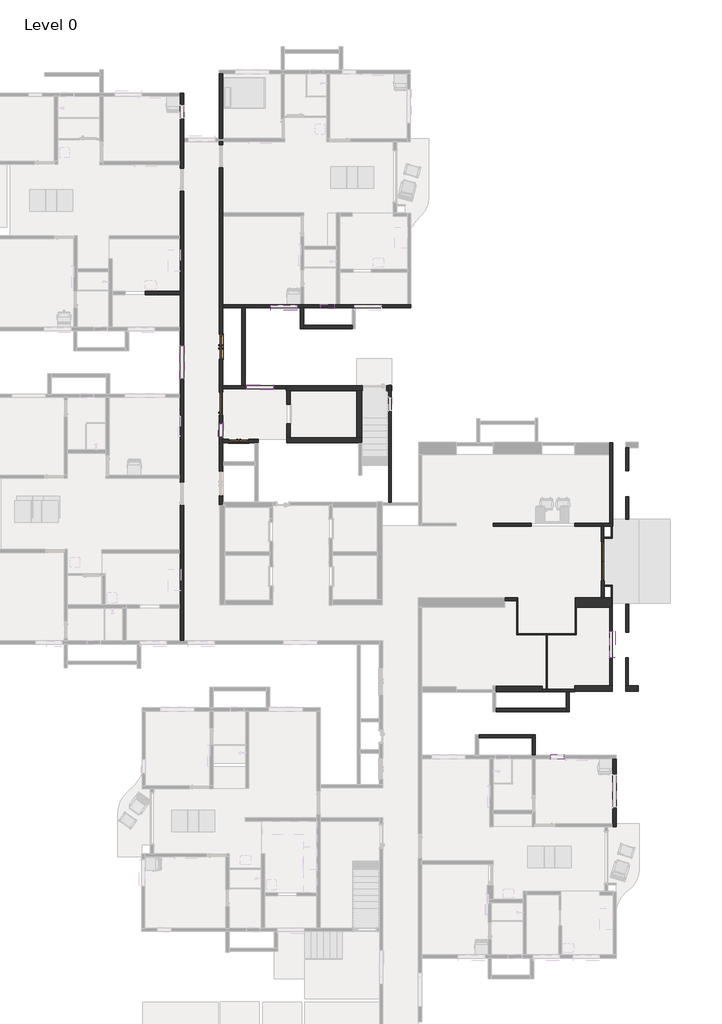
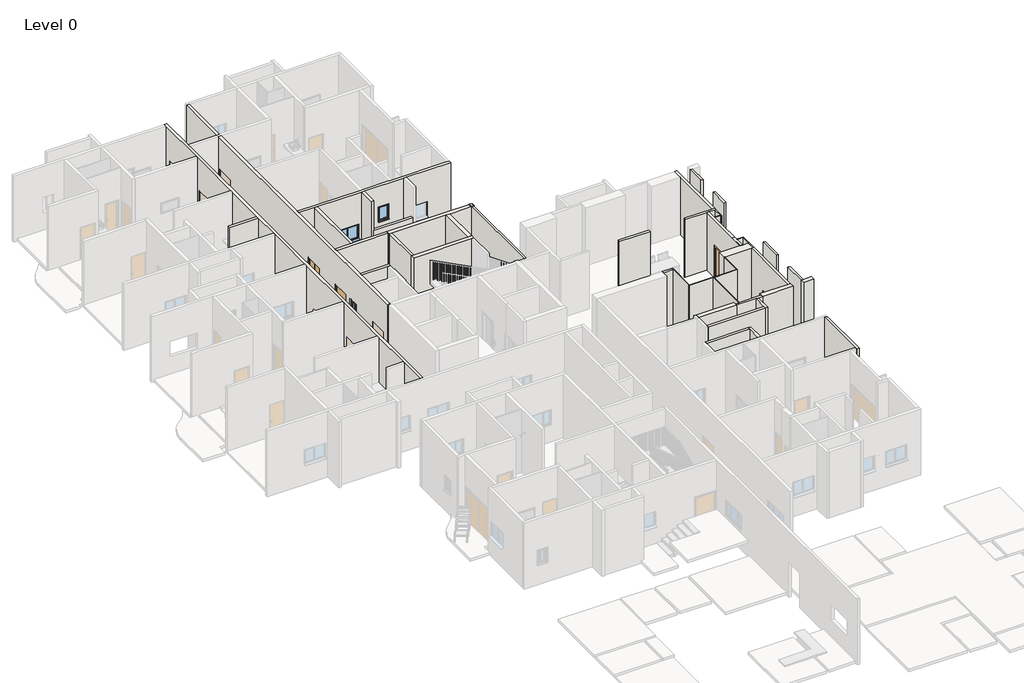
# One storey, part 6 of 14: 43 walls, 7 windows, 4 doors.
"""IFC4 building model written with IfcOpenShell, lengths in millimetres."""

from ifc_helpers import new_model, si_unit, frame, origin, origin_with_axes, place, context, project, spatial, polyline, outline, extrude, faceted_brep, transform, mapped, element, save
from components import doors_extdbl_flush_1810x2110mm_47ab578d, doors_extdbl_flush_3_b8e651f3, doors_extdbl_flush_3_75_39ca422f, doors_extsgl_flush_d1_30a970b5, windows_concept_plain_dbl_4_d1e2e333, windows_concept_plain_dbl_4_70a487c4, windows_sgl_plain_2_be143095, windows_tpl_variable_casement_2_47b04551, windows_tpl_variable_casement_4_346b9f46, windows_tpl_variable_casement_5_ffad3fa3

model = new_model("IFC4")

# Units and contexts
model_context = context("Model", 3, world=origin())
ifc_project = project(units=[si_unit("LENGTHUNIT", "METRE", prefix="MILLI")], contexts=[model_context])

# Site, building, storey
site = spatial("IfcSite", under=ifc_project)
building = spatial("IfcBuilding", under=site)
storey = spatial("IfcBuildingStorey", under=building, Name="Level 0", Elevation=0.0)

# Doors
placement = place(None, origin())
doors_extdbl_flush_1810x2110mm_shape = doors_extdbl_flush_1810x2110mm_47ab578d(model_context)
element("IfcDoor", 1, ObjectType="Doors_ExtDbl_Flush : 1810x2110mm", at=placement, inside=storey, context=model_context, shape_type="MappedRepresentation", body=[
    mapped(doors_extdbl_flush_1810x2110mm_shape, transform((-11411.1602598, 42923.0397358, 355.6), x_axis=(0.0, 1.0, 0.0), y_axis=(-1.0, 0.0, 0.0), z_axis=(0.0, 0.0, 1.0))),
])
doors_extdbl_flush_3_shape = doors_extdbl_flush_3_b8e651f3(model_context)
element("IfcDoor", 2, ObjectType="Doors_ExtDbl_Flush : 3'", at=placement, inside=storey, context=model_context, shape_type="MappedRepresentation", body=[
    mapped(doors_extdbl_flush_3_shape, transform((-28269.1280109, 48493.8706597, 0.0), x_axis=(-1.0, 0.0, 0.0), y_axis=(0.0, -1.0, 0.0), z_axis=(0.0, 0.0, 1.0))),
])
doors_extdbl_flush_3_75_shape = doors_extdbl_flush_3_75_39ca422f(model_context)
element("IfcDoor", 3, ObjectType="Doors_ExtDbl_Flush : 3.75'", at=placement, inside=storey, context=model_context, shape_type="MappedRepresentation", body=[
    mapped(doors_extdbl_flush_3_75_shape, transform((-29094.6788109, 52859.4702597, 0.0), x_axis=(0.0, -1.0, 0.0), y_axis=(1.0, 0.0, 0.0), z_axis=(0.0, 0.0, 1.0))),
])
doors_extsgl_flush_d1_shape = doors_extsgl_flush_d1_30a970b5(model_context)
element("IfcDoor", 4, ObjectType="Doors_ExtSgl_Flush : D1", at=placement, inside=storey, context=model_context, shape_type="MappedRepresentation", body=[
    mapped(doors_extsgl_flush_d1_shape, transform((-29094.6788109, 50221.0706597, 0.0), x_axis=(0.0, 1.0, 0.0), y_axis=(-1.0, 0.0, 0.0), z_axis=(0.0, 0.0, 1.0))),
])

# Walls
element("IfcWall", 5, ObjectType="W1", at=placement, inside=storey, context=model_context, shape_type="Brep", body=[
    faceted_brep([(-14673.0486976, 34891.8759386, 0.0), (-14673.0486976, 34739.4759386, 0.0), (-14673.0486976, 33939.3122683, 0.0), (-14673.0486976, 33939.3122683, 4000.0), (-14673.0486976, 34739.4759386, 4000.0), (-14673.0486976, 34891.8759386, 4000.0), (-14520.6486976, 34891.8759386, 0.0), (-14520.6486976, 34891.8759386, 4000.0), (-14520.6486976, 33939.3122683, 4000.0), (-14520.6486976, 33939.3122683, 0.0)], [[[0, 1, 2, 3, 4, 5]], [[6, 7, 8, 9]], [[2, 1, 0, 6, 9]], [[5, 4, 3, 8, 7]], [[3, 2, 9, 8]], [[0, 5, 7, 6]]]),
])
element("IfcWall", 6, ObjectType="W1", at=placement, inside=storey, context=model_context, shape_type="Brep", body=[
    faceted_brep([(-10935.2417798, 33786.9122683, 0.0), (-10935.2417798, 30776.9106683, 0.0), (-10935.2417798, 30624.5106683, 0.0), (-10935.2417798, 30624.5106683, 4000.0), (-10935.2417798, 30776.9106683, 4000.0), (-10935.2417798, 33786.9122683, 4000.0), (-10935.2417798, 33043.9114683, 2110.0), (-10935.2417798, 31519.9114683, 2110.0), (-10935.2417798, 31519.9114683, 1200.0), (-10935.2417798, 33043.9114683, 1200.0), (-10782.8417798, 33786.9122683, 0.0), (-10782.8417798, 33786.9122683, 4000.0), (-10782.8417798, 30624.5106683, 4000.0), (-10782.8417798, 30624.5106683, 0.0), (-10782.8417798, 33043.9114683, 2110.0), (-10782.8417798, 33043.9114683, 1200.0), (-10782.8417798, 31519.9114683, 1200.0), (-10782.8417798, 31519.9114683, 2110.0)], [[[0, 1, 2, 3, 4, 5], [6, 7, 8, 9]], [[10, 11, 12, 13], [14, 15, 16, 17]], [[2, 1, 0, 10, 13]], [[5, 4, 3, 12, 11]], [[0, 5, 11, 10]], [[3, 2, 13, 12]], [[15, 14, 6, 9]], [[16, 15, 9, 8]], [[17, 16, 8, 7]], [[14, 17, 7, 6]]]),
])
element("IfcWall", 7, ObjectType="W1", at=placement, inside=storey, context=model_context, shape_type="Brep", body=[
    faceted_brep([(-30819.9442282, 61132.2966557, 2110.0), (-30819.9442282, 61132.2966557, 0.0), (-30819.9442282, 62364.2982557, 0.0), (-30819.9442282, 62516.6982557, 0.0), (-30819.9442282, 64612.2998557, 0.0), (-30819.9442282, 64612.2998557, 4000.0), (-30819.9442282, 62516.6982557, 4000.0), (-30819.9442282, 62364.2982557, 4000.0), (-30819.9442282, 39237.6998557, 4000.0), (-30819.9442282, 39237.6998557, 0.0), (-30819.9442282, 45511.2966557, 0.0), (-30819.9442282, 45511.2966557, 2110.0), (-30819.9442282, 46578.0966557, 2110.0), (-30819.9442282, 46578.0966557, 0.0), (-30819.9442282, 60065.4966557, 0.0), (-30819.9442282, 60065.4966557, 2110.0), (-30819.9442282, 64053.4998557, 2110.0), (-30819.9442282, 64053.4998557, 1200.0), (-30819.9442282, 63443.8998557, 1200.0), (-30819.9442282, 63443.8998557, 2110.0), (-30819.9442282, 52902.8998557, 2110.0), (-30819.9442282, 52902.8998557, 1200.0), (-30819.9442282, 51378.8998557, 1200.0), (-30819.9442282, 51378.8998557, 2110.0), (-30972.3442282, 64612.2998557, 0.0), (-30972.3442282, 64459.8998557, 0.0), (-30972.3442282, 61449.8982557, 0.0), (-30972.3442282, 61297.4982557, 0.0), (-30972.3442282, 61132.2966557, 0.0), (-30972.3442282, 61132.2966557, 2110.0), (-30972.3442282, 60065.4966557, 2110.0), (-30972.3442282, 60065.4966557, 0.0), (-30972.3442282, 58008.2998557, 0.0), (-30972.3442282, 57855.8998557, 0.0), (-30972.3442282, 55424.4170169, 0.0), (-30972.3442282, 55272.0170169, 0.0), (-30972.3442282, 53766.4998557, 0.0), (-30972.3442282, 53614.0998557, 0.0), (-30972.3442282, 50667.6998557, 0.0), (-30972.3442282, 50515.2998557, 0.0), (-30972.3442282, 46921.0982557, 0.0), (-30972.3442282, 46768.6982557, 0.0), (-30972.3442282, 46578.0966557, 0.0), (-30972.3442282, 46578.0966557, 2110.0), (-30972.3442282, 45511.2966557, 2110.0), (-30972.3442282, 45511.2966557, 0.0), (-30972.3442282, 43460.4498557, 0.0), (-30972.3442282, 43308.0498557, 0.0), (-30972.3442282, 40908.6978471, 0.0), (-30972.3442282, 40756.2978471, 0.0), (-30972.3442282, 39237.6998557, 0.0), (-30972.3442282, 39237.6998557, 4000.0), (-30972.3442282, 40756.2978471, 4000.0), (-30972.3442282, 40908.6978471, 4000.0), (-30972.3442282, 43308.0498557, 4000.0), (-30972.3442282, 43460.4498557, 4000.0), (-30972.3442282, 46768.6982557, 4000.0), (-30972.3442282, 46921.0982557, 4000.0), (-30972.3442282, 50515.2998557, 4000.0), (-30972.3442282, 50667.6998557, 4000.0), (-30972.3442282, 53614.0998557, 4000.0), (-30972.3442282, 53766.4998557, 4000.0), (-30972.3442282, 55272.0170169, 4000.0), (-30972.3442282, 55424.4170169, 4000.0), (-30972.3442282, 57855.8998557, 4000.0), (-30972.3442282, 58008.2998557, 4000.0), (-30972.3442282, 61297.4982557, 4000.0), (-30972.3442282, 61449.8982557, 4000.0), (-30972.3442282, 64459.8998557, 4000.0), (-30972.3442282, 64612.2998557, 4000.0), (-30972.3442282, 64053.4998557, 2110.0), (-30972.3442282, 63443.8998557, 2110.0), (-30972.3442282, 63443.8998557, 1200.0), (-30972.3442282, 64053.4998557, 1200.0), (-30972.3442282, 52902.8998557, 2110.0), (-30972.3442282, 51378.8998557, 2110.0), (-30972.3442282, 51378.8998557, 1200.0), (-30972.3442282, 52902.8998557, 1200.0)], [[[0, 1, 2, 3, 4, 5, 6, 7, 8, 9, 10, 11, 12, 13, 14, 15], [16, 17, 18, 19], [20, 21, 22, 23]], [[24, 25, 26, 27, 28, 29, 30, 31, 32, 33, 34, 35, 36, 37, 38, 39, 40, 41, 42, 43, 44, 45, 46, 47, 48, 49, 50, 51, 52, 53, 54, 55, 56, 57, 58, 59, 60, 61, 62, 63, 64, 65, 66, 67, 68, 69], [70, 71, 72, 73], [74, 75, 76, 77]], [[10, 9, 50, 49, 48, 47, 46, 45]], [[14, 13, 42, 41, 40, 39, 38, 37, 36, 35, 34, 33, 32, 31]], [[4, 3, 2, 1, 28, 27, 26, 25, 24]], [[8, 7, 6, 5, 69, 68, 67, 66, 65, 64, 63, 62, 61, 60, 59, 58, 57, 56, 55, 54, 53, 52, 51]], [[9, 8, 51, 50]], [[5, 4, 24, 69]], [[45, 44, 11, 10]], [[43, 42, 13, 12]], [[44, 43, 12, 11]], [[31, 30, 15, 14]], [[29, 28, 1, 0]], [[30, 29, 0, 15]], [[17, 16, 70, 73]], [[18, 17, 73, 72]], [[19, 18, 72, 71]], [[16, 19, 71, 70]], [[21, 20, 74, 77]], [[22, 21, 77, 76]], [[23, 22, 76, 75]], [[20, 23, 75, 74]]]),
])
element("IfcWall", 8, ObjectType="W1", at=placement, inside=storey, context=model_context, shape_type="Brep", body=[
    faceted_brep([(-29170.8788109, 45547.3690597, 0.0), (-29170.8788109, 45547.3690597, 4000.0), (-29170.8788109, 62364.2982557, 4000.0), (-29170.8788109, 62364.2982557, 0.0), (-29170.8788109, 62212.0810361, 0.0), (-29170.8788109, 62212.0810361, 2110.0), (-29170.8788109, 61145.2810361, 2110.0), (-29170.8788109, 61145.2810361, 0.0), (-29170.8788109, 53430.9702597, 0.0), (-29170.8788109, 53430.9702597, 2110.0), (-29170.8788109, 52287.9702597, 2110.0), (-29170.8788109, 52287.9702597, 0.0), (-29170.8788109, 50754.4706597, 0.0), (-29170.8788109, 50754.4706597, 2110.0), (-29170.8788109, 49687.6706597, 2110.0), (-29170.8788109, 49687.6706597, 0.0), (-29170.8788109, 47096.8706597, 0.0), (-29170.8788109, 47096.8706597, 2110.0), (-29170.8788109, 45953.8706597, 2110.0), (-29170.8788109, 45953.8706597, 0.0), (-29170.8788109, 48697.0706597, 2110.0), (-29170.8788109, 48697.0706597, 1200.0), (-29170.8788109, 49306.6706597, 1200.0), (-29170.8788109, 49306.6706597, 2110.0), (-29018.4788109, 45547.3690597, 4000.0), (-29018.4788109, 45547.3690597, 0.0), (-29018.4788109, 45661.6690597, 0.0), (-29018.4788109, 45953.8706597, 0.0), (-29018.4788109, 45953.8706597, 2110.0), (-29018.4788109, 47096.8706597, 2110.0), (-29018.4788109, 47096.8706597, 0.0), (-29018.4788109, 47376.2706597, 0.0), (-29018.4788109, 47528.6706597, 0.0), (-29018.4788109, 48417.6706597, 0.0), (-29018.4788109, 48570.0706597, 0.0), (-29018.4788109, 49687.6706597, 0.0), (-29018.4788109, 49687.6706597, 2110.0), (-29018.4788109, 50754.4706597, 2110.0), (-29018.4788109, 50754.4706597, 0.0), (-29018.4788109, 50906.8706597, 0.0), (-29018.4788109, 51059.2706597, 0.0), (-29018.4788109, 52287.9702597, 0.0), (-29018.4788109, 52287.9702597, 2110.0), (-29018.4788109, 53430.9702597, 2110.0), (-29018.4788109, 53430.9702597, 0.0), (-29018.4788109, 54659.6698597, 0.0), (-29018.4788109, 54812.0698597, 0.0), (-29018.4788109, 58910.0810361, 0.0), (-29018.4788109, 59062.4810361, 0.0), (-29018.4788109, 61145.2810361, 0.0), (-29018.4788109, 61145.2810361, 2110.0), (-29018.4788109, 62212.0810361, 2110.0), (-29018.4788109, 62212.0810361, 0.0), (-29018.4788109, 62364.2982557, 0.0), (-29018.4788109, 62364.2982557, 4000.0), (-29018.4788109, 59062.4810361, 4000.0), (-29018.4788109, 58910.0810361, 4000.0), (-29018.4788109, 54812.0698597, 4000.0), (-29018.4788109, 54659.6698597, 4000.0), (-29018.4788109, 51059.2706597, 4000.0), (-29018.4788109, 50906.8706597, 4000.0), (-29018.4788109, 48570.0706597, 4000.0), (-29018.4788109, 48417.6706597, 4000.0), (-29018.4788109, 47528.6706597, 4000.0), (-29018.4788109, 47376.2706597, 4000.0), (-29018.4788109, 45661.6690597, 4000.0), (-29018.4788109, 48697.0706597, 1200.0), (-29018.4788109, 48697.0706597, 2110.0), (-29018.4788109, 49306.6706597, 2110.0), (-29018.4788109, 49306.6706597, 1200.0), (-29147.4805211, 45547.3690597, 0.0), (-29147.4805211, 45547.3690597, 4000.0)], [[[0, 1, 2, 3, 4, 5, 6, 7, 8, 9, 10, 11, 12, 13, 14, 15, 16, 17, 18, 19], [20, 21, 22, 23]], [[24, 25, 26, 27, 28, 29, 30, 31, 32, 33, 34, 35, 36, 37, 38, 39, 40, 41, 42, 43, 44, 45, 46, 47, 48, 49, 50, 51, 52, 53, 54, 55, 56, 57, 58, 59, 60, 61, 62, 63, 64, 65], [66, 67, 68, 69]], [[25, 70, 0, 19, 27, 26]], [[7, 49, 48, 47, 46, 45, 44, 8]], [[52, 4, 3, 53]], [[11, 41, 40, 39, 38, 12]], [[30, 16, 15, 35, 34, 33, 32, 31]], [[1, 0, 70, 25, 24, 71]], [[1, 71, 24, 65, 64, 63, 62, 61, 60, 59, 58, 57, 56, 55, 54, 2]], [[3, 2, 54, 53]], [[7, 6, 50, 49]], [[5, 4, 52, 51]], [[6, 5, 51, 50]], [[21, 20, 67, 66]], [[22, 21, 66, 69]], [[23, 22, 69, 68]], [[20, 23, 68, 67]], [[44, 43, 9, 8]], [[42, 41, 11, 10]], [[43, 42, 10, 9]], [[30, 29, 17, 16]], [[28, 27, 19, 18]], [[29, 28, 18, 17]], [[15, 14, 36, 35]], [[13, 12, 38, 37]], [[14, 13, 37, 36]]]),
    faceted_brep([(-29170.8788109, 65518.2714597, 4000.0), (-29170.8788109, 65518.2714597, 0.0), (-29170.8788109, 62516.6982557, 0.0), (-29170.8788109, 62516.6982557, 4000.0), (-29018.4788109, 65518.2714597, 0.0), (-29018.4788109, 65518.2714597, 4000.0), (-29018.4788109, 62516.6982557, 4000.0), (-29018.4788109, 62516.6982557, 0.0)], [[[0, 1, 2, 3]], [[4, 5, 6, 7]], [[1, 4, 7, 2]], [[5, 0, 3, 6]], [[1, 0, 5, 4]], [[3, 2, 7, 6]]]),
])
element("IfcWall", 9, ObjectType="W1", at=placement, inside=storey, context=model_context, shape_type="Brep", body=[
    faceted_brep([(-29018.4788109, 54659.6698597, 0.0), (-28116.6772109, 54659.6698597, 0.0), (-27964.2772109, 54659.6698597, 0.0), (-25411.6788109, 54659.6698597, 0.0), (-25259.2788109, 54659.6698597, 0.0), (-23011.2772109, 54659.6698597, 0.0), (-22858.8772109, 54659.6698597, 0.0), (-20293.4772109, 54659.6698597, 0.0), (-20293.4772109, 54659.6698597, 4000.0), (-22858.8772109, 54659.6698597, 4000.0), (-23011.2772109, 54659.6698597, 4000.0), (-25259.2788109, 54659.6698597, 4000.0), (-25411.6788109, 54659.6698597, 4000.0), (-27964.2772109, 54659.6698597, 4000.0), (-28116.6772109, 54659.6698597, 4000.0), (-29018.4788109, 54659.6698597, 4000.0), (-21665.0772109, 54659.6698597, 2110.0), (-21665.0772109, 54659.6698597, 1200.0), (-22884.2772109, 54659.6698597, 1200.0), (-22884.2772109, 54659.6698597, 2110.0), (-25564.0788109, 54659.6698597, 2110.0), (-25564.0788109, 54659.6698597, 1200.0), (-26783.2788109, 54659.6698597, 1200.0), (-26783.2788109, 54659.6698597, 2110.0), (-23849.4772109, 54659.6698597, 2738.9328), (-23849.4772109, 54659.6698597, 1828.9328), (-24459.0772109, 54659.6698597, 1828.9328), (-24459.0772109, 54659.6698597, 2738.9328), (-29018.4788109, 54812.0698597, 0.0), (-29018.4788109, 54812.0698597, 4000.0), (-25398.8772109, 54812.0698597, 4000.0), (-25246.4772109, 54812.0698597, 4000.0), (-23747.8772109, 54812.0698597, 4000.0), (-23595.4772109, 54812.0698597, 4000.0), (-20445.8772109, 54812.0698597, 4000.0), (-20293.4772109, 54812.0698597, 4000.0), (-20293.4772109, 54812.0698597, 0.0), (-20445.8772109, 54812.0698597, 0.0), (-23595.4772109, 54812.0698597, 0.0), (-23747.8772109, 54812.0698597, 0.0), (-25246.4772109, 54812.0698597, 0.0), (-25398.8772109, 54812.0698597, 0.0), (-21665.0772109, 54812.0698597, 2110.0), (-22884.2772109, 54812.0698597, 2110.0), (-22884.2772109, 54812.0698597, 1200.0), (-21665.0772109, 54812.0698597, 1200.0), (-25564.0788109, 54812.0698597, 2110.0), (-26783.2788109, 54812.0698597, 2110.0), (-26783.2788109, 54812.0698597, 1200.0), (-25564.0788109, 54812.0698597, 1200.0), (-23849.4772109, 54812.0698597, 2738.9328), (-24459.0772109, 54812.0698597, 2738.9328), (-24459.0772109, 54812.0698597, 1828.9328), (-23849.4772109, 54812.0698597, 1828.9328)], [[[0, 1, 2, 3, 4, 5, 6, 7, 8, 9, 10, 11, 12, 13, 14, 15], [16, 17, 18, 19], [20, 21, 22, 23], [24, 25, 26, 27]], [[28, 29, 30, 31, 32, 33, 34, 35, 36, 37, 38, 39, 40, 41], [42, 43, 44, 45], [46, 47, 48, 49], [50, 51, 52, 53]], [[7, 6, 5, 4, 3, 2, 1, 0, 28, 41, 40, 39, 38, 37, 36]], [[15, 14, 13, 12, 11, 10, 9, 8, 35, 34, 33, 32, 31, 30, 29]], [[0, 15, 29, 28]], [[8, 7, 36, 35]], [[17, 16, 42, 45]], [[18, 17, 45, 44]], [[19, 18, 44, 43]], [[16, 19, 43, 42]], [[21, 20, 46, 49]], [[22, 21, 49, 48]], [[23, 22, 48, 47]], [[20, 23, 47, 46]], [[25, 24, 50, 53]], [[26, 25, 53, 52]], [[27, 26, 52, 51]], [[24, 27, 51, 50]]]),
])
element("IfcWall", 10, ObjectType="W1", at=placement, inside=storey, context=model_context, shape_type="Brep", body=[
    faceted_brep([(-25411.6788109, 54659.6698597, 0.0), (-25411.6788109, 53707.0682597, 0.0), (-25411.6788109, 53707.0682597, 4000.0), (-25411.6788109, 54659.6698597, 4000.0), (-25259.2788109, 54659.6698597, 0.0), (-25259.2788109, 54659.6698597, 4000.0), (-25259.2788109, 53707.0682597, 4000.0), (-25259.2788109, 53707.0682597, 2171.2), (-25259.2788109, 53707.0682597, 0.0), (-25259.2788109, 53859.4682597, 0.0)], [[[0, 1, 2, 3]], [[4, 5, 6, 7, 8, 9]], [[1, 0, 4, 9, 8]], [[3, 2, 6, 5]], [[0, 3, 5, 4]], [[2, 1, 8, 7, 6]]]),
])
element("IfcWall", 11, ObjectType="W1", at=placement, inside=storey, context=model_context, shape_type="SweptSolid", body=[
    extrude(outline(polyline([(-28116.6772109, 51059.2706597), (-28116.6772109, 54659.6698597), (-27964.2772109, 54659.6698597), (-27964.2772109, 51059.2706597), (-28116.6772109, 51059.2706597)])), origin_with_axes(), (0.0, 0.0, 1.0), 4000.0),
])
element("IfcWall", 12, ObjectType="W1", at=placement, inside=storey, context=model_context, shape_type="Brep", body=[
    faceted_brep([(-29018.4788109, 50906.8706597, 0.0), (-26059.2772109, 50906.8706597, 0.0), (-26059.2772109, 50906.8706597, 4000.0), (-29018.4788109, 50906.8706597, 4000.0), (-27888.0772109, 50906.8706597, 2110.0), (-26668.8772109, 50906.8706597, 2110.0), (-26668.8772109, 50906.8706597, 1200.0), (-27888.0772109, 50906.8706597, 1200.0), (-29018.4788109, 51059.2706597, 0.0), (-29018.4788109, 51059.2706597, 4000.0), (-28116.6772109, 51059.2706597, 4000.0), (-27964.2772109, 51059.2706597, 4000.0), (-26059.2772109, 51059.2706597, 4000.0), (-26059.2772109, 51059.2706597, 0.0), (-27964.2772109, 51059.2706597, 0.0), (-28116.6772109, 51059.2706597, 0.0), (-27888.0772109, 51059.2706597, 2110.0), (-27888.0772109, 51059.2706597, 1200.0), (-26668.8772109, 51059.2706597, 1200.0), (-26668.8772109, 51059.2706597, 2110.0)], [[[0, 1, 2, 3], [4, 5, 6, 7]], [[8, 9, 10, 11, 12, 13, 14, 15], [16, 17, 18, 19]], [[1, 0, 8, 15, 14, 13]], [[2, 1, 13, 12]], [[3, 2, 12, 11, 10, 9]], [[0, 3, 9, 8]], [[17, 16, 4, 7]], [[18, 17, 7, 6]], [[19, 18, 6, 5]], [[16, 19, 5, 4]]]),
])
element("IfcWall", 13, ObjectType="W1", at=placement, inside=storey, context=model_context, shape_type="Brep", body=[
    faceted_brep([(-29018.4788109, 48417.6706597, 0.0), (-28726.3280109, 48417.6706597, 0.0), (-28726.3280109, 48417.6706597, 2110.0), (-27811.9280109, 48417.6706597, 2110.0), (-27811.9280109, 48417.6706597, 0.0), (-27519.7772109, 48417.6706597, 0.0), (-27367.3772109, 48417.6706597, 0.0), (-27367.3772109, 48417.6706597, 4000.0), (-27519.7772109, 48417.6706597, 4000.0), (-29018.4788109, 48417.6706597, 4000.0), (-28726.3280109, 48570.0706597, 2110.0), (-28726.3280109, 48570.0706597, 0.0), (-29018.4788109, 48570.0706597, 0.0), (-29018.4788109, 48570.0706597, 4000.0), (-27367.3772109, 48570.0706597, 4000.0), (-27367.3772109, 48570.0706597, 0.0), (-27811.9280109, 48570.0706597, 0.0), (-27811.9280109, 48570.0706597, 2110.0)], [[[0, 1, 2, 3, 4, 5, 6, 7, 8, 9]], [[10, 11, 12, 13, 14, 15, 16, 17]], [[16, 15, 6, 5, 4]], [[12, 11, 1, 0]], [[9, 8, 7, 14, 13]], [[0, 9, 13, 12]], [[7, 6, 15, 14]], [[4, 3, 17, 16]], [[2, 1, 11, 10]], [[3, 2, 10, 17]]]),
])
element("IfcWall", 14, ObjectType="W1", at=placement, inside=storey, context=model_context, shape_type="SweptSolid", body=[
    extrude(outline(polyline([(48652.2320599, 4000.0), (50830.6706597, 4000.0), (50830.6706597, 0.0), (50191.4513598, 0.0), (50191.4513598, 2100.0), (49291.4513598, 2100.0), (49291.4513598, 0.0), (48652.2320599, 0.0), (48652.2320599, 4000.0)])), frame((-26039.7911684, 0.0, 0.0), z_axis=(1.0, 0.0, 0.0), x_axis=(0.0, 1.0, 0.0)), (0.0, 0.0, 1.0), 152.4),
])
element("IfcWall", 15, ObjectType="W1", at=placement, inside=storey, context=model_context, shape_type="SweptSolid", body=[
    extrude(outline(polyline([(-32602.2679937, 55424.4170169), (-30972.3442282, 55424.4170169), (-30972.3442282, 55272.0170169), (-32602.2679937, 55272.0170169), (-32602.2679937, 55424.4170169)])), origin_with_axes(), (0.0, 0.0, 1.0), 4000.0),
])
element("IfcWall", 16, ObjectType="W1", at=placement, inside=storey, context=model_context, shape_type="SweptSolid", body=[
    extrude(outline(polyline([(-25259.2788109, 53859.4682597), (-23011.2772109, 53859.4682597), (-23011.2772109, 53707.0682597), (-25259.2788109, 53707.0682597), (-25259.2788109, 53859.4682597)])), origin_with_axes(), (0.0, 0.0, 1.0), 2171.2),
])
element("IfcWall", 17, ObjectType="W1", at=placement, inside=storey, context=model_context, shape_type="SweptSolid", body=[
    extrude(outline(polyline([(-14673.0486976, 34739.4759386), (-17149.6502976, 34739.4759386), (-17149.6502976, 34891.8759386), (-14673.0486976, 34891.8759386), (-14673.0486976, 34739.4759386)])), origin_with_axes(), (0.0, 0.0, 1.0), 4000.0),
])
element("IfcWall", 18, ObjectType="W1", at=placement, inside=storey, context=model_context, shape_type="SweptSolid", body=[
    extrude(outline(polyline([(-13084.848117, 35955.4247386), (-16364.3901798, 35955.4247386), (-16364.3901798, 36107.8247386), (-13084.848117, 36107.8247386), (-13084.848117, 35955.4247386)])), origin_with_axes(), (0.0, 0.0, 1.0), 4000.0),
])
element("IfcWall", 19, ObjectType="W2", at=placement, inside=storey, context=model_context, shape_type="Brep", body=[
    faceted_brep([(-15396.146517, 39512.5147554, 0.0), (-14016.774117, 39512.5147554, 0.0), (-13967.396517, 39512.5147554, 0.0), (-12627.546517, 39512.5147554, 0.0), (-12627.546517, 39512.5147554, 4000.0), (-13967.396517, 39512.5147554, 4000.0), (-14016.774117, 39512.5147554, 4000.0), (-15396.146517, 39512.5147554, 4000.0), (-15396.146517, 39561.8923554, 0.0), (-15396.146517, 39561.8923554, 4000.0), (-15346.768917, 39561.8923554, 4000.0), (-12676.924117, 39561.8923554, 4000.0), (-12627.546517, 39561.8923554, 4000.0), (-12627.546517, 39561.8923554, 0.0), (-12676.924117, 39561.8923554, 0.0), (-15346.768917, 39561.8923554, 0.0)], [[[0, 1, 2, 3, 4, 5, 6, 7]], [[8, 9, 10, 11, 12, 13, 14, 15]], [[3, 2, 1, 0, 8, 15, 14, 13]], [[7, 6, 5, 4, 12, 11, 10, 9]], [[0, 7, 9, 8]], [[4, 3, 13, 12]]]),
])
element("IfcWall", 20, ObjectType="W2", at=placement, inside=storey, context=model_context, shape_type="Brep", body=[
    faceted_brep([(-15346.768917, 39561.8923554, 0.0), (-15346.768917, 41238.2923554, 0.0), (-15346.768917, 41238.2923554, 4000.0), (-15346.768917, 39561.8923554, 4000.0), (-15396.146517, 39561.8923554, 0.0), (-15396.146517, 39561.8923554, 4000.0), (-15396.146517, 41107.636729, 4000.0), (-15396.146517, 41234.738329, 4000.0), (-15396.146517, 41238.2923554, 4000.0), (-15396.146517, 41238.2923554, 0.0), (-15396.146517, 41234.738329, 0.0), (-15396.146517, 41107.636729, 0.0)], [[[0, 1, 2, 3]], [[4, 5, 6, 7, 8, 9, 10, 11]], [[1, 0, 4, 11, 10, 9]], [[2, 1, 9, 8]], [[3, 2, 8, 7, 6, 5]], [[0, 3, 5, 4]]]),
])
element("IfcWall", 21, ObjectType="W2", at=placement, inside=storey, context=model_context, shape_type="SweptSolid", body=[
    extrude(outline(polyline([(-14016.774117, 37003.2763386), (-14016.774117, 39512.5147554), (-13967.396517, 39512.5147554), (-13967.396517, 37003.2763386), (-14016.774117, 37003.2763386)])), origin_with_axes(), (0.0, 0.0, 1.0), 4000.0),
])
element("IfcWall", 22, ObjectType="W2", at=placement, inside=storey, context=model_context, shape_type="SweptSolid", body=[
    extrude(outline(polyline([(-12627.546517, 40794.2677015), (-12627.546517, 39561.8923554), (-12676.924117, 39561.8923554), (-12676.924117, 40794.2677015), (-12627.546517, 40794.2677015)])), origin_with_axes(), (0.0, 0.0, 1.0), 4000.0),
])
element("IfcWall", 23, ObjectType="W2", at=placement, inside=storey, context=model_context, shape_type="Brep", body=[
    faceted_brep([(-11009.6370598, 44555.1147358, 0.0), (-11009.6370598, 44029.8173358, 0.0), (-11009.6370598, 43980.4397358, 0.0), (-11009.6370598, 43980.4397358, 4000.0), (-11009.6370598, 44029.8173358, 4000.0), (-11009.6370598, 44555.1147358, 4000.0), (-10960.2594598, 44555.1147358, 0.0), (-10960.2594598, 44555.1147358, 4000.0), (-10960.2594598, 43980.4397358, 4000.0), (-10960.2594598, 43980.4397358, 0.0)], [[[0, 1, 2, 3, 4, 5]], [[6, 7, 8, 9]], [[2, 1, 0, 6, 9]], [[5, 4, 3, 8, 7]], [[0, 5, 7, 6]], [[3, 2, 9, 8]]]),
])
element("IfcWall", 24, ObjectType="W2", at=placement, inside=storey, context=model_context, shape_type="SweptSolid", body=[
    extrude(outline(polyline([(-11347.6094598, 44029.8173358), (-11009.6370598, 44029.8173358), (-11009.6370598, 43980.4397358), (-11347.6094598, 43980.4397358), (-11347.6094598, 44029.8173358)])), origin_with_axes(), (0.0, 0.0, 1.0), 4000.0),
])
element("IfcWall", 25, ObjectType="W2", at=placement, inside=storey, context=model_context, shape_type="Brep", body=[
    faceted_brep([(-11345.1194566, 41773.029377, 0.0), (-11013.4970566, 41773.029377, 0.0), (-10964.1194566, 41773.029377, 0.0), (-10964.1194566, 41773.029377, 4000.0), (-11013.4970566, 41773.029377, 4000.0), (-11345.1194566, 41773.029377, 4000.0), (-11345.1194566, 41822.406977, 0.0), (-11345.1194566, 41822.406977, 4000.0), (-10964.1194566, 41822.406977, 4000.0), (-10964.1194566, 41822.406977, 0.0)], [[[0, 1, 2, 3, 4, 5]], [[6, 7, 8, 9]], [[2, 1, 0, 6, 9]], [[5, 4, 3, 8, 7]], [[0, 5, 7, 6]], [[3, 2, 9, 8]]]),
])
element("IfcWall", 26, ObjectType="W2", at=placement, inside=storey, context=model_context, shape_type="Brep", body=[
    faceted_brep([(-11013.4970566, 41773.029377, 0.0), (-11013.4970566, 41232.5701015, 0.0), (-11013.4970566, 40794.2677015, 0.0), (-11013.4970566, 40794.2677015, 4000.0), (-11013.4970566, 41232.5701015, 4000.0), (-11013.4970566, 41773.029377, 4000.0), (-10964.1194566, 41773.029377, 0.0), (-10964.1194566, 41773.029377, 4000.0), (-10964.1194566, 40794.2677015, 4000.0), (-10964.1194566, 40794.2677015, 0.0)], [[[0, 1, 2, 3, 4, 5]], [[6, 7, 8, 9]], [[2, 1, 0, 6, 9]], [[5, 4, 3, 8, 7]], [[0, 5, 7, 6]], [[3, 2, 9, 8]]]),
])
element("IfcWall", 27, ObjectType="W3", at=placement, inside=storey, context=model_context, shape_type="Brep", body=[
    faceted_brep([(-12706.8917798, 36898.5267386, 0.0), (-10954.2917798, 36898.5267386, 0.0), (-10954.2917798, 36898.5267386, 4000.0), (-12706.8917798, 36898.5267386, 4000.0), (-12706.8917798, 37158.8259386, 0.0), (-12706.8917798, 37158.8259386, 4000.0), (-11081.3933798, 37158.8259386, 4000.0), (-10954.2917798, 37158.8259386, 4000.0), (-10954.2917798, 37158.8259386, 0.0), (-11081.3933798, 37158.8259386, 0.0), (-12706.8917798, 37003.2763386, 0.0), (-12706.8917798, 37003.2763386, 4000.0)], [[[0, 1, 2, 3]], [[4, 5, 6, 7, 8, 9]], [[1, 0, 10, 4, 9, 8]], [[3, 2, 7, 6, 5, 11]], [[0, 3, 11, 5, 4, 10]], [[2, 1, 8, 7]]]),
])
element("IfcWall", 28, ObjectType="W3", at=placement, inside=storey, context=model_context, shape_type="Brep", body=[
    faceted_brep([(-16364.3901798, 36873.1267386, 0.0), (-14205.4917798, 36873.1267386, 0.0), (-14205.4917798, 36873.1267386, 4000.0), (-16364.3901798, 36873.1267386, 4000.0), (-16364.3901798, 37133.4259386, 0.0), (-16364.3901798, 37133.4259386, 4000.0), (-14205.4917798, 37133.4259386, 4000.0), (-14205.4917798, 37133.4259386, 0.0), (-14205.4917798, 37003.2763386, 0.0), (-14205.4917798, 36876.1747386, 0.0), (-14205.4917798, 37003.2763386, 4000.0), (-14205.4917798, 36876.1747386, 4000.0)], [[[0, 1, 2, 3]], [[4, 5, 6, 7]], [[1, 0, 4, 7, 8, 9]], [[2, 1, 9, 8, 7, 6, 10, 11]], [[3, 2, 11, 10, 6, 5]], [[0, 3, 5, 4]]]),
])
element("IfcWall", 29, ObjectType="W3", at=placement, inside=storey, context=model_context, shape_type="Brep", body=[
    faceted_brep([(-9760.4917798, 37158.8259386, 0.0), (-10217.5901798, 37158.8259386, 0.0), (-10344.6917798, 37158.8259386, 0.0), (-10344.6917798, 37158.8259386, 4000.0), (-10217.5901798, 37158.8259386, 4000.0), (-9760.4917798, 37158.8259386, 4000.0), (-9760.4917798, 36898.5267386, 0.0), (-9760.4917798, 36898.5267386, 4000.0), (-10344.6917798, 36898.5267386, 4000.0), (-10344.6917798, 36898.5267386, 0.0)], [[[0, 1, 2, 3, 4, 5]], [[6, 7, 8, 9]], [[2, 1, 0, 6, 9]], [[5, 4, 3, 8, 7]], [[0, 5, 7, 6]], [[3, 2, 9, 8]]]),
])
element("IfcWall", 30, ObjectType="W5", at=placement, inside=storey, context=model_context, shape_type="Brep", body=[
    faceted_brep([(-26039.7911684, 48423.6320599, 0.0), (-22706.5788109, 48423.6320599, 0.0), (-22579.4772109, 48423.6320599, 0.0), (-22579.4772109, 48423.6320599, 4000.0), (-22706.5788109, 48423.6320599, 4000.0), (-26039.7911684, 48423.6320599, 4000.0), (-26039.7911684, 48652.2320599, 0.0), (-26039.7911684, 48652.2320599, 4000.0), (-25887.3911684, 48652.2320599, 4000.0), (-22808.0772109, 48652.2320599, 4000.0), (-22579.4772109, 48652.2320599, 4000.0), (-22579.4772109, 48652.2320599, 0.0), (-22808.0772109, 48652.2320599, 0.0), (-25887.3911684, 48652.2320599, 0.0)], [[[0, 1, 2, 3, 4, 5]], [[6, 7, 8, 9, 10, 11, 12, 13]], [[2, 1, 0, 6, 13, 12, 11]], [[5, 4, 3, 10, 9, 8, 7]], [[3, 2, 11, 10]], [[0, 5, 7, 6]]]),
])
element("IfcWall", 31, ObjectType="W5", at=placement, inside=storey, context=model_context, shape_type="Brep", body=[
    faceted_brep([(-21167.4288686, 50830.6706597, 0.0), (-21167.4288686, 50830.6706597, 4000.0), (-22579.4772109, 50830.6706597, 4000.0), (-22808.0772109, 50830.6706597, 4000.0), (-25887.3911684, 50830.6706597, 4000.0), (-26039.7911684, 50830.6706597, 4000.0), (-26059.2772109, 50830.6706597, 4000.0), (-26059.2772109, 50830.6706597, 0.0), (-26039.7911684, 50830.6706597, 0.0), (-25887.3911684, 50830.6706597, 0.0), (-22808.0772109, 50830.6706597, 0.0), (-22579.4772109, 50830.6706597, 0.0), (-22554.0772109, 50830.6706597, 0.0), (-22554.0772109, 50830.6706597, 2133.6), (-21411.0772109, 50830.6706597, 2133.6), (-21411.0772109, 50830.6706597, 0.0), (-21167.4288686, 51059.2706597, 4000.0), (-21167.4288686, 51059.2706597, 0.0), (-21411.0772109, 51059.2706597, 0.0), (-21411.0772109, 51059.2706597, 2133.6), (-22554.0772109, 51059.2706597, 2133.6), (-22554.0772109, 51059.2706597, 0.0), (-26059.2772109, 51059.2706597, 0.0), (-26059.2772109, 51059.2706597, 4000.0), (-26059.2772109, 50906.8706597, 0.0), (-26059.2772109, 50906.8706597, 4000.0)], [[[0, 1, 2, 3, 4, 5, 6, 7, 8, 9, 10, 11, 12, 13, 14, 15]], [[16, 17, 18, 19, 20, 21, 22, 23]], [[17, 0, 15, 18]], [[7, 24, 22, 21, 12, 11, 10, 9, 8]], [[1, 0, 17, 16]], [[6, 5, 4, 3, 2, 1, 16, 23, 25]], [[7, 6, 25, 23, 22, 24]], [[20, 13, 12, 21]], [[13, 20, 19, 14]], [[14, 19, 18, 15]]]),
])
element("IfcWall", 32, ObjectType="W5", at=placement, inside=storey, context=model_context, shape_type="SweptSolid", body=[
    extrude(outline(polyline([(-22808.0772109, 48652.2320599), (-22808.0772109, 50830.6706597), (-22579.4772109, 50830.6706597), (-22579.4772109, 48652.2320599), (-22808.0772109, 48652.2320599)])), origin_with_axes(), (0.0, 0.0, 1.0), 4000.0),
])
element("IfcWall", 33, ObjectType="W6", at=placement, inside=storey, context=model_context, shape_type="Brep", body=[
    faceted_brep([(-21319.9304686, 51084.5182597, 0.0), (-21319.9304686, 51045.185879, 0.0), (-21319.9304686, 50918.084279, 0.0), (-21319.9304686, 45636.2690597, 0.0), (-21319.9304686, 45636.2690597, 4000.0), (-21319.9304686, 50918.084279, 4000.0), (-21319.9304686, 51045.185879, 4000.0), (-21319.9304686, 51084.5182597, 4000.0), (-21319.9304686, 50511.684279, 2110.0), (-21319.9304686, 49902.084279, 2110.0), (-21319.9304686, 49902.084279, 1200.0), (-21319.9304686, 50511.684279, 1200.0), (-21192.8288686, 51084.5182597, 0.0), (-21192.8288686, 51084.5182597, 4000.0), (-21192.8288686, 45636.2690597, 4000.0), (-21192.8288686, 45636.2690597, 0.0), (-21192.8288686, 50511.684279, 2110.0), (-21192.8288686, 50511.684279, 1200.0), (-21192.8288686, 49902.084279, 1200.0), (-21192.8288686, 49902.084279, 2110.0)], [[[0, 1, 2, 3, 4, 5, 6, 7], [8, 9, 10, 11]], [[12, 13, 14, 15], [16, 17, 18, 19]], [[3, 2, 1, 0, 12, 15]], [[7, 6, 5, 4, 14, 13]], [[0, 7, 13, 12]], [[4, 3, 15, 14]], [[17, 16, 8, 11]], [[18, 17, 11, 10]], [[19, 18, 10, 9]], [[16, 19, 9, 8]]]),
])
element("IfcWall", 34, ObjectType="W6", at=placement, inside=storey, context=model_context, shape_type="Brep", body=[
    faceted_brep([(-14205.4917798, 36876.1747386, 0.0), (-13084.848117, 36876.1747386, 0.0), (-12957.746517, 36876.1747386, 0.0), (-12706.8917798, 36876.1747386, 0.0), (-12706.8917798, 36876.1747386, 4000.0), (-12957.746517, 36876.1747386, 4000.0), (-13084.848117, 36876.1747386, 4000.0), (-14205.4917798, 36876.1747386, 4000.0), (-14205.4917798, 37003.2763386, 0.0), (-14205.4917798, 37003.2763386, 4000.0), (-14016.774117, 37003.2763386, 4000.0), (-13967.396517, 37003.2763386, 4000.0), (-12706.8917798, 37003.2763386, 4000.0), (-12706.8917798, 37003.2763386, 0.0), (-13967.396517, 37003.2763386, 0.0), (-14016.774117, 37003.2763386, 0.0), (-12706.8917798, 36898.5267386, 0.0), (-12706.8917798, 36898.5267386, 4000.0)], [[[0, 1, 2, 3, 4, 5, 6, 7]], [[8, 9, 10, 11, 12, 13, 14, 15]], [[3, 2, 1, 0, 8, 15, 14, 13, 16]], [[4, 3, 16, 13, 12, 17]], [[7, 6, 5, 4, 17, 12, 11, 10, 9]], [[0, 7, 9, 8]]]),
])
element("IfcWall", 35, ObjectType="W6", at=placement, inside=storey, context=model_context, shape_type="Brep", body=[
    faceted_brep([(-13084.848117, 36876.1747386, 0.0), (-13084.848117, 36107.8247386, 0.0), (-13084.848117, 35955.4247386, 0.0), (-13084.848117, 35955.4247386, 4000.0), (-13084.848117, 36107.8247386, 4000.0), (-13084.848117, 36876.1747386, 4000.0), (-12957.746517, 36876.1747386, 0.0), (-12957.746517, 36876.1747386, 4000.0), (-12957.746517, 35955.4247386, 4000.0), (-12957.746517, 35955.4247386, 0.0)], [[[0, 1, 2, 3, 4, 5]], [[6, 7, 8, 9]], [[2, 1, 0, 6, 9]], [[5, 4, 3, 8, 7]], [[0, 5, 7, 6]], [[3, 2, 9, 8]]]),
])
element("IfcWall", 36, ObjectType="W6", at=placement, inside=storey, context=model_context, shape_type="Brep", body=[
    faceted_brep([(-10954.2917798, 37158.8259386, 0.0), (-10954.2917798, 40794.2677015, 0.0), (-10954.2917798, 40794.2677015, 4000.0), (-10954.2917798, 37158.8259386, 4000.0), (-10954.2917798, 39676.6677015, 2110.0), (-10954.2917798, 39676.6677015, 1200.0), (-10954.2917798, 38457.4677015, 1200.0), (-10954.2917798, 38457.4677015, 2110.0), (-11081.3933798, 37158.8259386, 0.0), (-11081.3933798, 37158.8259386, 4000.0), (-11081.3933798, 40794.2677015, 4000.0), (-11081.3933798, 40794.2677015, 0.0), (-11081.3933798, 39676.6677015, 2110.0), (-11081.3933798, 38457.4677015, 2110.0), (-11081.3933798, 38457.4677015, 1200.0), (-11081.3933798, 39676.6677015, 1200.0), (-11013.4970566, 40794.2677015, 0.0), (-10964.1194566, 40794.2677015, 0.0), (-10964.1194566, 40794.2677015, 4000.0), (-11013.4970566, 40794.2677015, 4000.0)], [[[0, 1, 2, 3], [4, 5, 6, 7]], [[8, 9, 10, 11], [12, 13, 14, 15]], [[1, 0, 8, 11, 16, 17]], [[3, 2, 18, 19, 10, 9]], [[0, 3, 9, 8]], [[2, 1, 17, 16, 11, 10, 19, 18]], [[5, 4, 12, 15]], [[6, 5, 15, 14]], [[7, 6, 14, 13]], [[4, 7, 13, 12]]]),
])
element("IfcWall", 37, ObjectType="W6", at=placement, inside=storey, context=model_context, shape_type="SweptSolid", body=[
    extrude(outline(polyline([(-14727.0872405, 44551.7207072), (-16479.6872405, 44551.7207072), (-16479.6872405, 44678.8223072), (-14727.0872405, 44678.8223072), (-14727.0872405, 44551.7207072)])), origin_with_axes(), (0.0, 0.0, 1.0), 4000.0),
])
element("IfcWall", 38, ObjectType="W6", at=placement, inside=storey, context=model_context, shape_type="Brep", body=[
    faceted_brep([(-12693.8094598, 44555.1147358, 0.0), (-11474.7110598, 44555.1147358, 0.0), (-11347.6094598, 44555.1147358, 0.0), (-11009.6370598, 44555.1147358, 0.0), (-10960.2594598, 44555.1147358, 0.0), (-10947.5594598, 44555.1147358, 0.0), (-10947.5594598, 44555.1147358, 4000.0), (-10960.2594598, 44555.1147358, 4000.0), (-11009.6370598, 44555.1147358, 4000.0), (-11347.6094598, 44555.1147358, 4000.0), (-11474.7110598, 44555.1147358, 4000.0), (-12693.8094598, 44555.1147358, 4000.0), (-12693.8094598, 44682.2163358, 0.0), (-12693.8094598, 44682.2163358, 4000.0), (-11074.6610598, 44682.2163358, 4000.0), (-10947.5594598, 44682.2163358, 4000.0), (-10947.5594598, 44682.2163358, 0.0), (-11074.6610598, 44682.2163358, 0.0)], [[[0, 1, 2, 3, 4, 5, 6, 7, 8, 9, 10, 11]], [[12, 13, 14, 15, 16, 17]], [[5, 4, 3, 2, 1, 0, 12, 17, 16]], [[11, 10, 9, 8, 7, 6, 15, 14, 13]], [[0, 11, 13, 12]], [[6, 5, 16, 15]]]),
])
element("IfcWall", 39, ObjectType="W6", at=placement, inside=storey, context=model_context, shape_type="Brep", body=[
    faceted_brep([(-11474.7110598, 44555.1147358, 0.0), (-11474.7110598, 41265.8655358, 0.0), (-11474.7110598, 41265.8655358, 4000.0), (-11474.7110598, 44555.1147358, 4000.0), (-11474.7110598, 42018.0397358, 2465.6), (-11474.7110598, 42018.0397358, 355.6), (-11474.7110598, 43828.0397358, 355.6), (-11474.7110598, 43828.0397358, 2465.6), (-11347.6094598, 44555.1147358, 0.0), (-11347.6094598, 44555.1147358, 4000.0), (-11347.6094598, 44029.8173358, 4000.0), (-11347.6094598, 43980.4397358, 4000.0), (-11347.6094598, 41265.8655358, 4000.0), (-11347.6094598, 41265.8655358, 0.0), (-11347.6094598, 43980.4397358, 0.0), (-11347.6094598, 44029.8173358, 0.0), (-11347.6094598, 42018.0397358, 2465.6), (-11347.6094598, 43828.0397358, 2465.6), (-11347.6094598, 43828.0397358, 355.6), (-11347.6094598, 42018.0397358, 355.6)], [[[0, 1, 2, 3], [4, 5, 6, 7]], [[8, 9, 10, 11, 12, 13, 14, 15], [16, 17, 18, 19]], [[1, 0, 8, 15, 14, 13]], [[2, 1, 13, 12]], [[3, 2, 12, 11, 10, 9]], [[0, 3, 9, 8]], [[5, 4, 16, 19]], [[6, 5, 19, 18]], [[7, 6, 18, 17]], [[4, 7, 17, 16]]]),
])
element("IfcWall", 40, ObjectType="W6", at=placement, inside=storey, context=model_context, shape_type="Brep", body=[
    faceted_brep([(-10947.5594598, 44682.2163358, 0.0), (-10947.5594598, 48426.9165308, 0.0), (-10947.5594598, 48426.9165308, 4000.0), (-10947.5594598, 44682.2163358, 4000.0), (-11074.6610598, 44682.2163358, 0.0), (-11074.6610598, 44682.2163358, 4000.0), (-11074.6610598, 47868.2181308, 4000.0), (-11074.6610598, 48426.9165308, 4000.0), (-11074.6610598, 48426.9165308, 0.0), (-11074.6610598, 47868.2181308, 0.0)], [[[0, 1, 2, 3]], [[4, 5, 6, 7, 8, 9]], [[1, 0, 4, 9, 8]], [[3, 2, 7, 6, 5]], [[0, 3, 5, 4]], [[2, 1, 8, 7]]]),
])
element("IfcWall", 41, ObjectType="W6", at=placement, inside=storey, context=model_context, shape_type="SweptSolid", body=[
    extrude(outline(polyline([(-10332.1242051, 39640.9027936), (-10332.1242051, 40936.3027936), (-10205.0226051, 40936.3027936), (-10205.0226051, 39640.9027936), (-10332.1242051, 39640.9027936)])), origin_with_axes(), (0.0, 0.0, 1.0), 4000.0),
])
element("IfcWall", 42, ObjectType="W6", at=placement, inside=storey, context=model_context, shape_type="SweptSolid", body=[
    extrude(outline(polyline([(-10217.5901798, 38454.2259386), (-10217.5901798, 37158.8259386), (-10344.6917798, 37158.8259386), (-10344.6917798, 38454.2259386), (-10217.5901798, 38454.2259386)])), origin_with_axes(), (0.0, 0.0, 1.0), 4000.0),
])
element("IfcWall", 43, ObjectType="W6", at=placement, inside=storey, context=model_context, shape_type="SweptSolid", body=[
    extrude(outline(polyline([(-10201.6129289, 45916.8031635), (-10201.6129289, 44862.7031635), (-10328.7145289, 44862.7031635), (-10328.7145289, 45916.8031635), (-10201.6129289, 45916.8031635)])), origin_with_axes(), (0.0, 0.0, 1.0), 4000.0),
])
element("IfcWall", 44, ObjectType="W6", at=placement, inside=storey, context=model_context, shape_type="SweptSolid", body=[
    extrude(outline(polyline([(-10201.6129289, 48181.1171358), (-10201.6129289, 47120.6163358), (-10328.7145289, 47120.6163358), (-10328.7145289, 48181.1171358), (-10201.6129289, 48181.1171358)])), origin_with_axes(), (0.0, 0.0, 1.0), 4000.0),
])
element("IfcWall", 45, ObjectType="W6", at=placement, inside=storey, context=model_context, shape_type="Brep", body=[
    faceted_brep([(-11472.2210566, 42012.906977, 0.0), (-11472.2210566, 41232.5701015, 0.0), (-11472.2210566, 41232.5701015, 4000.0), (-11472.2210566, 42012.906977, 4000.0), (-11345.1194566, 42012.906977, 0.0), (-11345.1194566, 42012.906977, 4000.0), (-11345.1194566, 41822.406977, 4000.0), (-11345.1194566, 41773.029377, 4000.0), (-11345.1194566, 41232.5701015, 4000.0), (-11345.1194566, 41232.5701015, 0.0), (-11345.1194566, 41773.029377, 0.0), (-11345.1194566, 41822.406977, 0.0)], [[[0, 1, 2, 3]], [[4, 5, 6, 7, 8, 9, 10, 11]], [[1, 0, 4, 11, 10, 9]], [[3, 2, 8, 7, 6, 5]], [[0, 3, 5, 4]], [[2, 1, 9, 8]]]),
])
element("IfcWall", 46, ObjectType="W6", at=placement, inside=storey, context=model_context, shape_type="SweptSolid", body=[
    extrude(outline(polyline([(-15396.146517, 41107.636729), (-15945.4745014, 41107.636729), (-15945.4745014, 41234.738329), (-15396.146517, 41234.738329), (-15396.146517, 41107.636729)])), origin_with_axes(), (0.0, 0.0, 1.0), 4000.0),
])
element("IfcWall", 47, ObjectType="W8", at=placement, inside=storey, context=model_context, shape_type="Brep", body=[
    faceted_brep([(-12685.7638897, 40794.2677015, 0.0), (-12676.924117, 40794.2677015, 0.0), (-12627.546517, 40794.2677015, 0.0), (-11081.3933798, 40794.2677015, 0.0), (-11013.4970566, 40794.2677015, 0.0), (-11013.4970566, 40794.2677015, 4000.0), (-11081.3933798, 40794.2677015, 4000.0), (-12627.546517, 40794.2677015, 4000.0), (-12676.924117, 40794.2677015, 4000.0), (-12685.7638897, 40794.2677015, 4000.0), (-12685.7638897, 41232.5701015, 0.0), (-12685.7638897, 41232.5701015, 4000.0), (-11472.2210566, 41232.5701015, 4000.0), (-11345.1194566, 41232.5701015, 4000.0), (-11013.4970566, 41232.5701015, 4000.0), (-11013.4970566, 41232.5701015, 0.0), (-11345.1194566, 41232.5701015, 0.0), (-11472.2210566, 41232.5701015, 0.0)], [[[0, 1, 2, 3, 4, 5, 6, 7, 8, 9]], [[10, 11, 12, 13, 14, 15, 16, 17]], [[4, 3, 2, 1, 0, 10, 17, 16, 15]], [[9, 8, 7, 6, 5, 14, 13, 12, 11]], [[0, 9, 11, 10]], [[5, 4, 15, 14]]]),
])

# Windows
windows_concept_plain_dbl_4_shape = windows_concept_plain_dbl_4_d1e2e333(model_context)
element("IfcWindow", 48, ObjectType="Windows_Concept_Plain_Dbl : 4'", at=placement, inside=storey, context=model_context, shape_type="MappedRepresentation", body=[
    mapped(windows_concept_plain_dbl_4_shape, transform((-26458.6788109, 54744.3264275, 0.0), x_axis=(-1.0, 0.0, 0.0), y_axis=(0.0, -1.0, 0.0), z_axis=(0.0, 0.0, 1.0))),
])
windows_concept_plain_dbl_4_2_shape = windows_concept_plain_dbl_4_70a487c4(model_context)
element("IfcWindow", 49, ObjectType="Windows_Concept_Plain_Dbl : 4'", at=placement, inside=storey, context=model_context, shape_type="MappedRepresentation", body=[
    mapped(windows_concept_plain_dbl_4_2_shape, transform((-11026.2991476, 38782.0677015, 0.0), x_axis=(0.0, -1.0, 0.0), y_axis=(1.0, 0.0, 0.0), z_axis=(0.0, 0.0, 1.0))),
])
windows_sgl_plain_2_shape = windows_sgl_plain_2_be143095(model_context)
element("IfcWindow", 50, ObjectType="Windows_Sgl_Plain : 2'", at=placement, inside=storey, context=model_context, shape_type="MappedRepresentation", body=[
    mapped(windows_sgl_plain_2_shape, transform((-24154.2772109, 54744.3264275, 628.9328), x_axis=(-1.0, 0.0, 0.0), y_axis=(0.0, -1.0, 0.0), z_axis=(0.0, 0.0, 1.0))),
])
windows_tpl_variable_casement_2_shape = windows_tpl_variable_casement_2_47b04551(model_context)
element("IfcWindow", 51, ObjectType="Windows_Tpl_Variable_Casement : 2'", at=placement, inside=storey, context=model_context, shape_type="MappedRepresentation", body=[
    mapped(windows_tpl_variable_casement_2_shape, transform((-13514.8486976, 33854.6557005, 0.0), x_axis=(1.0, 0.0, 0.0), y_axis=(0.0, 1.0, 0.0), z_axis=(0.0, 0.0, 1.0))),
])
element("IfcWindow", 52, ObjectType="Windows_Tpl_Variable_Casement : 2'", at=placement, inside=storey, context=model_context, shape_type="MappedRepresentation", body=[
    mapped(windows_tpl_variable_casement_2_shape, transform((-29086.2222431, 48991.6706597, 0.0), x_axis=(0.0, 1.0, 0.0), y_axis=(-1.0, 0.0, 0.0), z_axis=(0.0, 0.0, 1.0))),
])
windows_tpl_variable_casement_4_shape = windows_tpl_variable_casement_4_346b9f46(model_context)
element("IfcWindow", 53, ObjectType="Windows_Tpl_Variable_Casement : 4'", at=placement, inside=storey, context=model_context, shape_type="MappedRepresentation", body=[
    mapped(windows_tpl_variable_casement_4_shape, transform((-26983.8772109, 50974.6140919, 0.0), x_axis=(1.0, 0.0, 0.0), y_axis=(0.0, 1.0, 0.0), z_axis=(0.0, 0.0, 1.0))),
])
windows_tpl_variable_casement_5_shape = windows_tpl_variable_casement_5_ffad3fa3(model_context)
element("IfcWindow", 54, ObjectType="Windows_Tpl_Variable_Casement : 5'", at=placement, inside=storey, context=model_context, shape_type="MappedRepresentation", body=[
    mapped(windows_tpl_variable_casement_5_shape, transform((-30904.600796, 51693.8998557, 0.0), x_axis=(0.0, -1.0, 0.0), y_axis=(1.0, 0.0, 0.0), z_axis=(0.0, 0.0, 1.0))),
])

save(model, "model.ifc")

# Revit data of these elements
# Type "Doors_ExtDbl_Flush : 1810x2110mm"
#   Type Mark = "44"
#   Type Comments = "External Double"
#   Operation = "DoubleDoorSingleSwing"
#   Keynote = "L20"
#   Analytic Construction = "Metal"
#   Wrap Layers (Ext) from Ext = 102.5 mm
#   Wrap Layers (Int) from Ext = 177.5 mm
#   Thickness = 44 mm
#   Rough Width = 1810 mm
#   Rough Height = 2110 mm
#   O/A Frame Width = 64 mm
#   Heat Transfer Coefficient (U) = 3.7021 W/(m²·K)
#   Handle Z Distance = 1050 mm
#   FrameWidth = 42 mm
#   FrameOffset - External = 25 mm
#   FrameDepth = 89 mm
#   Door Panel Width = 852 mm
#   Door Panel Thickness = 44 mm
#   Door Panel Height = 2000 mm
#   Cill Thickness = 54.5 mm
#   Cill Projection = 30 mm
#   Handle X Distance = 75 mm
#   Height = 2110 mm
#   Structural Tolerance = 6.5 mm
#   Tolerance = 3 mm
#   Undercut = 4 mm
#   Width = 1810 mm
#   Cill Extension = 25 mm
#   Cavity Closer Width = 50 mm
#   Cavity Closer Offset from Ext = 102.5 mm
#   Cavity Closer Depth = 85 mm
#   Define Thermal Properties by = 0
#   Vis - Ironmongery = yes
#   Vis - Cavity Closers = yes
#   Function = 1
#   Material Door = Door - Panel
#   Material Frame = Door - Frame/Mullion
#   Material Ironmongery = Door - Handle
#   Visual Light Transmittance = 0
#   Thermal Resistance (R) = 0
#   Solar Heat Gain Coefficient = 0
#   Wall Closure = (empty or 0)
# Type "Doors_ExtDbl_Flush : 3'"
#   Type Mark = "55"
#   Type Comments = "External Double"
#   Operation = "DoubleDoorSingleSwing"
#   Keynote = "L20"
#   Analytic Construction = "Metal"
#   Wrap Layers (Ext) from Ext = 102.5 mm
#   Wrap Layers (Int) from Ext = 177.5 mm
#   Thickness = 44 mm
#   Rough Width = 914.4 mm
#   Rough Height = 2110 mm
#   O/A Frame Width = 64 mm
#   Heat Transfer Coefficient (U) = 3.7021 W/(m²·K)
#   Handle Z Distance = 1050 mm
#   FrameWidth = 42 mm
#   FrameOffset - External = 25 mm
#   FrameDepth = 89 mm
#   Door Panel Width = 404.2 mm
#   Door Panel Thickness = 44 mm
#   Door Panel Height = 2000 mm
#   Cill Thickness = 54.5 mm
#   Cill Projection = 30 mm
#   Handle X Distance = 75 mm
#   Height = 2110 mm
#   Structural Tolerance = 6.5 mm
#   Tolerance = 3 mm
#   Undercut = 4 mm
#   Width = 914.4 mm
#   Cill Extension = 25 mm
#   Cavity Closer Width = 50 mm
#   Cavity Closer Offset from Ext = 102.5 mm
#   Cavity Closer Depth = 85 mm
#   Vis - Ironmongery = yes
#   Vis - Cavity Closers = yes
#   Function = 1
#   Material Door = Door - Panel
#   Material Frame = Door - Frame/Mullion
#   Material Ironmongery = Door - Handle
#   Visual Light Transmittance = 0
#   Thermal Resistance (R) = 0
#   Solar Heat Gain Coefficient = 0
#   Wall Closure = (empty or 0)
# Type "Doors_ExtDbl_Flush : 3.75'"
#   Type Mark = "54"
#   Type Comments = "External Double"
#   Operation = "DoubleDoorSingleSwing"
#   Keynote = "L20"
#   Analytic Construction = "Metal"
#   Wrap Layers (Ext) from Ext = 102.5 mm
#   Wrap Layers (Int) from Ext = 177.5 mm
#   Thickness = 44 mm
#   Rough Width = 1143 mm
#   Rough Height = 2110 mm
#   O/A Frame Width = 64 mm
#   Heat Transfer Coefficient (U) = 3.7021 W/(m²·K)
#   Handle Z Distance = 1050 mm
#   FrameWidth = 42 mm
#   FrameOffset - External = 25 mm
#   FrameDepth = 89 mm
#   Door Panel Width = 518.5 mm
#   Door Panel Thickness = 44 mm
#   Door Panel Height = 2000 mm
#   Cill Thickness = 54.5 mm
#   Cill Projection = 30 mm
#   Handle X Distance = 75 mm
#   Height = 2110 mm
#   Structural Tolerance = 6.5 mm
#   Tolerance = 3 mm
#   Undercut = 4 mm
#   Width = 1143 mm
#   Cill Extension = 25 mm
#   Cavity Closer Width = 50 mm
#   Cavity Closer Offset from Ext = 102.5 mm
#   Cavity Closer Depth = 85 mm
#   Vis - Ironmongery = yes
#   Vis - Cavity Closers = yes
#   Function = 1
#   Material Door = Door - Panel
#   Material Frame = Door - Frame/Mullion
#   Material Ironmongery = Door - Handle
#   Visual Light Transmittance = 0
#   Thermal Resistance (R) = 0
#   Solar Heat Gain Coefficient = 0
#   Wall Closure = (empty or 0)
# Type "Doors_ExtSgl_Flush : D1"
#   Type Mark = "49"
#   Type Comments = "External Single"
#   Operation = "SingleSwingRight"
#   Construction Type Id = "MDOOR"
#   Keynote = "L20"
#   Analytic Construction = "Metal"
#   Wrap Layers (Int) from Ext = 177.5 mm
#   Wrap Layers (Ext) from Ext = 102.5 mm
#   Thickness = 44 mm
#   Rough Width = 1066.8 mm
#   Rough Height = 2110 mm
#   O/A Frame Width = 64 mm
#   Heat Transfer Coefficient (U) = 3.7021 W/(m²·K)
#   Handle Z Distance = 1050 mm
#   FrameWidth = 42 mm
#   FrameOffset - External = 25 mm
#   FrameDepth = 89 mm
#   Door Panel Width = 963.8 mm
#   Door Panel Thickness = 44 mm
#   Door Panel Height = 2000 mm
#   Cill Thickness = 54.5 mm
#   Cill Projection = 30 mm
#   Handle X Distance = 75 mm
#   Height = 2110 mm
#   Structural Tolerance = 6.5 mm
#   Tolerance = 3 mm
#   Undercut = 4 mm
#   Width = 1066.8 mm
#   Cill Extension = 25 mm
#   Cavity Closer Width = 50 mm
#   Cavity Closer Offset from Ext = 102.5 mm
#   Cavity Closer Depth = 85 mm
#   Vis - Ironmongery = yes
#   Vis - Cavity Closers = yes
#   Define Thermal Properties by = 1
#   Function = 1
#   Material Door = Door - Panel
#   Material Frame = Door - Frame/Mullion
#   Material Ironmongery = Door - Handle
#   Visual Light Transmittance = 0
#   Solar Heat Gain Coefficient = 0
#   Wall Closure = (empty or 0)
# Type "W1"
#   Keynote = "F10"
#   Layers, outside or top first: 152.4 mm "Brick, Common" (function 1)
# Type "W2"
#   Keynote = "F10"
#   Layers, outside or top first: 49.378 mm "Brick, Common" (function 1)
# Type "W3"
#   Keynote = "F10"
#   Layers, outside or top first: 260.299 mm "Brick, Common" (function 1)
# Type "W5"
#   Keynote = "F10"
#   Layers, outside or top first: 228.6 mm "Brick, Common" (function 1)
# Type "W6"
#   Keynote = "F10"
#   Layers, outside or top first: 127.102 mm "Brick, Common" (function 1)
# Type "W8"
#   Keynote = "F10"
#   Layers, outside or top first: 438.302 mm "Brick, Common" (function 1)
# Type "Windows_Concept_Plain_Dbl : 4'"
#   Type Mark = "56"
#   Operation = "DoublePanelVertical"
#   Construction Type Id = "GSP4R"
#   Manufacturer = "Revit"
#   Keynote = "L10"
#   Analytic Construction = "1/8 in Pilkington single glazing"
#   Visual Light Transmittance = 0.9
#   Solar Heat Gain Coefficient = 0.78
#   Rough Width = 1219.2 mm
#   Rough Height = 910 mm
#   Height = 910 mm
#   Width = 1219.2 mm
#   Heat Transfer Coefficient (U) = 3.6886 W/(m²·K)
#   FrameOffset - External = 50 mm
#   Default Head Height = 2110 mm
#   Vis - Cavity Closers = yes
#   Define Thermal Properties by = 1
#   Material Trim = Window Frame
#   Material Glass = Glass
#   Material Frame = Window Frame
#   Wall Closure = (empty or 0)
# Type "Windows_Sgl_Plain : 2'"
#   Type Mark = "72"
#   Operation = "SinglePanel"
#   Construction Type Id = "SGL"
#   Manufacturer = "Revit"
#   Keynote = "L10"
#   Analytic Construction = "Large single-glazed windows"
#   Wrap Layers (Ext) from Ext = 102.5 mm
#   Wrap Layers (Int) from Ext = 177.5 mm
#   Window Board Projection = 25 mm
#   Window Board Extension = 25 mm
#   Visual Light Transmittance = 0.9
#   Solar Heat Gain Coefficient = 0.86
#   Rough Width = 609.6 mm
#   Rough Height = 910 mm
#   Height = 910 mm
#   Width = 609.6 mm
#   Heat Transfer Coefficient (U) = 5.5617 W/(m²·K)
#   Glazing Thickness = 24 mm
#   FrameOffset - External = 50 mm
#   Frame Depth = 65 mm
#   Default Head Height = 2110 mm
#   Cill Depth = 87.5 mm
#   Cavity Closer Width = 50 mm
#   Cavity Closer Offset from Ext = 102.5 mm
#   Cavity Closer Depth = 85 mm
#   Vis - Cavity Closers = yes
#   Define Thermal Properties by = 1
#   Material Trim = Window Frame
#   Material Glass = Glass
#   Material Frame = Window Frame
#   Wall Closure = (empty or 0)
# Type "Windows_Tpl_Variable_Casement : 2'"
#   Type Mark = "82"
#   Operation = "TriplePanelVertical"
#   Construction Type Id = "GSP4R"
#   Manufacturer = "Revit"
#   Keynote = "L10"
